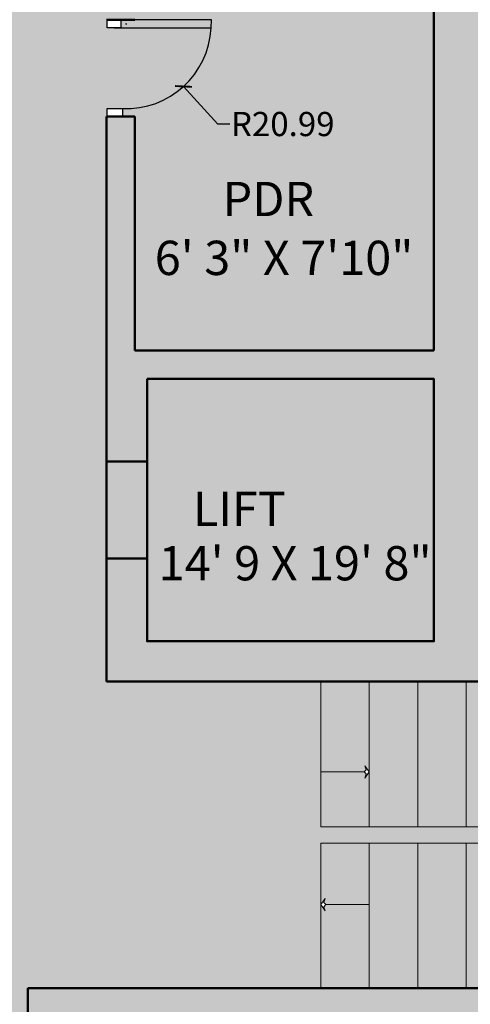
# Model space of a CAD drawing. Units: inches. Extents: x 925 to 2834, y 111 to 1355.
# Tile 7 of 25: x 1490 to 1602, y 638 to 882. Entities that reach past the tile are written whole.
import ezdxf

# ---------------------------------------------------------------- set-up
doc = ezdxf.new("R2010")
doc.units = ezdxf.units.IN
doc.header["$MEASUREMENT"] = 0
for name, color, linetype, lineweight in [('A-ANNO-DIMS', 2, 'Continuous', 18), ('A-AREA-IDEN', 7, 'Continuous', 18), ('A-DOOR', 2, 'Continuous', 25), ('A-FLOR-PATT', 252, 'Continuous', 13), ('A-FLOR-STRS', 4, 'Continuous', 18), ('A-WALL', 7, 'Continuous', 50), ('A-WALL-PATT', 8, 'Continuous', 13)]:
    doc.layers.add(name, color=color, linetype=linetype, lineweight=lineweight)
doc.styles.get("Standard").update_dxf_attribs({"font": 'arial.ttf'})
doc.dimstyles.get("Standard").update_dxf_attribs({"dimtxt": 6, "dimasz": 3, "dimexe": 0.18, "dimexo": 0.0625, "dimgap": 0.09, "dimtad": 0, "dimtih": 1, "dimtoh": 1, "dimdec": 1, "dimzin": 0, "dimdsep": 46, "dimlunit": 3, "dimtxsty": 'Standard', "dimblk": 'ARCHTICK', "dimcen": 0.09, "dimadec": 0, "dimazin": 0, "dimtfac": 1, "dimtdec": 1, "dimtofl": 0, "dimtmove": 0, "dimatfit": 3, "dimfxl": 1, "dimtolj": 1, "dimtzin": 0, "dimarcsym": 0})

# ---------------------------------------------------------------- blocks, each defined once
blk = doc.blocks.new('_ArchTick')
at = {"color": 0, "linetype": 'ByBlock', "const_width": 0.15}
blk.add_lwpolyline([(-0.5, -0.5), (0.5, 0.5)], dxfattribs=at)
blk = doc.blocks.new('*D83')
at = {"layer": 'A-ANNO-DIMS', "color": 0, "lineweight": -2, "transparency": 16777216}
for p, q in [((1516.5, 880.55), (1516.68, 880.55)), ((1516.59, 880.46), (1516.59, 880.64)), ((1539.21, 855.74), (1530.73, 865.05)), ((1542.21, 855.74), (1539.21, 855.74))]:
    blk.add_line(p, q, dxfattribs=at)
at = {"layer": 'Defpoints', "color": 0, "transparency": 16777216}
for p in [(1516.59, 880.55), (1530.73, 865.05)]:
    blk.add_point(p, dxfattribs=at)
at = {"layer": 'A-ANNO-DIMS', "color": 0, "lineweight": -2, "transparency": 16777216, "xscale": 3, "yscale": 3, "zscale": 3, "rotation": 132.3610318704431}
blk.add_blockref('_ArchTick', (1530.73, 865.05), dxfattribs=at)
at = {"layer": 'A-ANNO-DIMS', "color": 0, "transparency": 16777216, "insert": (1555.3, 855.74), "char_height": 6, "attachment_point": 5}
blk.add_mtext('\\A1;R20.99', dxfattribs=at)

msp = doc.modelspace()

# ---------------------------------------------------------------- hatches: boundary and pattern name
at = {"layer": 'A-FLOR-PATT', "transparency": 33554605}
h = msp.add_hatch(color=256, dxfattribs=at)
h.dxf.hatch_style = 1
h.paths.add_polyline_path([(1931.688, 1294.5638), (991.7375, 1294.5638), (991.7375, 172.1134), (1931.688, 172.1134)])
h.paths.add_polyline_path([(1910.7128, 1273.5886), (1910.7128, 193.0886), (1012.7128, 193.0886), (1012.7128, 1273.5886)], flags=16)
h.paths.add_polyline_path([(1850.7128, 1213.5886), (1850.7128, 253.0886), (1072.7128, 253.0886), (1072.7128, 1213.5886)], flags=0)
h.paths.add_polyline_path([(1838.7128, 1201.5886), (1838.7128, 265.0886), (1084.7128, 265.0886), (1084.7128, 530.5886), (1084.7128, 1201.5886)], flags=0)
h.paths.add_polyline_path([(1547.6758, 1155.7396), (1547.6758, 1119.115), (1513.0687, 1119.115), (1513.0687, 1155.7396)], flags=0)
h.paths.add_polyline_path([(1600.1067, 1154.9439), (1634.7139, 1154.9439), (1634.7139, 1119.115), (1600.1067, 1119.115)], flags=0)
h.paths.add_polyline_path([(1505.2502, 1144.5358), (1505.2502, 1119.115), (1470.643, 1119.115), (1470.643, 1144.5358)], flags=0)
h.paths.add_polyline_path([(1559.1357, 1141.0962), (1593.7428, 1141.0962), (1593.7428, 1119.115), (1559.1357, 1119.115)], flags=0)
h.paths.add_polyline_path([(1462.8966, 1154.9439), (1462.8966, 1119.115), (1428.2895, 1119.115), (1428.2895, 1154.9439)], flags=0)
h.paths.add_polyline_path([(1642.4603, 1144.5358), (1677.0675, 1144.5358), (1677.0675, 1119.115), (1642.4603, 1119.115)], flags=0)
h.paths.add_polyline_path([(1422.3508, 1141.0962), (1422.3508, 1119.115), (1387.7436, 1119.115), (1387.7436, 1141.0962)], flags=0)
h.paths.add_polyline_path([(1684.8859, 1155.7396), (1719.4931, 1155.7396), (1719.4931, 1119.115), (1684.8859, 1119.115)], flags=0)
h.paths.add_polyline_path([(1718.7128, 1081.5886), (1718.7128, 1050.1249), (1715.7128, 1050.1249), (1715.7128, 1026.1249), (1715.7128, 1002.1249), (1718.7128, 1002.1249), (1730.7128, 1002.1249), (1730.7128, 998.1249), (1730.7128, 990.1249), (1730.7128, 986.1249), (1718.7128, 986.1249), (1718.7128, 893.5886), (1715.3735, 893.5886), (1715.3735, 891.5886), (1713.3735, 891.5886, 0.41421356), (1677.3735, 855.5886), (1713.3735, 855.5886), (1713.3735, 853.5886), (1715.3735, 853.5886), (1715.3735, 851.5886), (1718.7128, 851.5886), (1718.7128, 821.5865), (1734.4655, 821.5865), (1734.3735, 819.5886, -0.41421356), (1712.4415, 793.5886), (1712.4415, 791.5886), (1718.7128, 791.5886), (1718.7128, 717.5886), (1718.7128, 669.5886), (1732.7128, 669.5886), (1732.7128, 665.5886), (1732.7128, 641.5886), (1732.7128, 634.5886), (1732.7128, 610.5886), (1732.7128, 603.5886), (1718.7128, 603.5886), (1718.7128, 385.0886), (1434.2128, 385.0886), (1434.2128, 530.5886), (1410.2128, 530.5886), (1408.2128, 530.5886), (1408.2128, 532.5886, 0.41421356), (1372.2128, 568.5886), (1372.2128, 532.5886), (1370.2128, 532.5886), (1370.2128, 530.5886), (1368.2128, 530.5886), (1282.2128, 530.5886), (1210.2128, 530.5886), (1200.2128, 530.5886), (1200.2128, 542.1915), (1183.2307, 542.1915), (1183.2307, 546.1915), (1200.2128, 546.1915), (1200.2128, 572.1915), (1183.2307, 572.1915), (1183.2307, 576.1915), (1200.2128, 576.1915), (1200.2128, 727.5886), (1210.2128, 727.5886), (1234.2128, 727.5886), (1259.7128, 727.5886), (1259.7128, 775.5886), (1259.7128, 799.5886), (1259.7128, 847.5886), (1259.7128, 993.5872), (1259.7128, 1065.5872), (1259.7128, 1071.5886), (1219.6318, 1071.5886), (1219.6318, 1081.5886), (1084.7128, 1081.5886), (1084.7128, 1119.115), (1256.8974, 1119.115), (1256.8974, 1154.9439), (1291.5046, 1154.9439), (1291.5046, 1119.115), (1256.8974, 1119.115), (1256.6723, 1081.5886), (1293.7128, 1081.5886), (1341.7128, 1081.5886), (1341.7128, 1093.5886), (1347.7128, 1093.5886), (1371.7128, 1093.5886), (1377.7128, 1093.5886), (1377.7128, 1081.5886), (1668.7128, 1081.5886), (1668.7128, 1117.5886), (1675.7128, 1117.5886), (1711.7128, 1117.5886), (1718.7128, 1117.5886)], flags=0)
h.paths.add_polyline_path([(1376.2838, 1155.7396), (1376.2838, 1119.115), (1341.6766, 1119.115), (1341.6766, 1155.7396)], flags=0)
h.paths.add_polyline_path([(1341.7128, 1076.0886), (1293.7128, 1076.0886), (1293.7128, 1071.5886), (1269.7128, 1071.5886), (1269.7128, 1065.5872), (1266.7128, 1065.5872), (1266.7128, 1029.5872), (1265.7128, 1029.5872), (1265.7128, 993.5872), (1269.7128, 993.5872), (1269.7128, 903.5886), (1269.7128, 893.5886), (1269.7128, 847.5886), (1265.2128, 847.5886), (1265.2128, 799.5886), (1269.7128, 799.5886), (1269.7128, 775.5886), (1265.2128, 775.5886), (1265.2128, 727.5886), (1269.7128, 727.5886), (1444.2128, 727.5886), (1444.2128, 717.5886), (1234.2128, 717.5886), (1234.2128, 722.0886), (1210.2128, 722.0886), (1210.2128, 717.5886), (1210.2128, 540.5886), (1210.2128, 536.0886), (1282.2128, 536.0886), (1282.2128, 535.0886), (1210.2128, 535.0886), (1210.2128, 540.5886), (1210.2128, 717.5886), (1210.2128, 723.0886), (1234.2128, 723.0886), (1234.2128, 717.5886), (1444.2128, 717.5886), (1444.2128, 727.5886), (1269.7128, 727.5886), (1264.2128, 727.5886), (1264.2128, 775.5886), (1269.7128, 775.5886), (1269.7128, 799.5886), (1264.2128, 799.5886), (1264.2128, 847.5886), (1269.7128, 847.5886), (1269.7128, 893.5886), (1269.7128, 903.5886), (1269.7128, 993.5872), (1264.7128, 993.5872), (1264.7128, 1029.5872), (1265.7128, 1029.5872), (1265.7128, 1065.5872), (1269.7128, 1065.5872), (1269.7128, 1071.5886), (1293.7128, 1071.5886), (1293.7128, 1077.0886), (1341.7128, 1077.0886)], flags=0)
h.paths.add_polyline_path([(1730.9529, 1141.0962), (1765.5601, 1141.0962), (1765.5601, 1119.115), (1730.9529, 1119.115)], flags=0)
h.paths.add_polyline_path([(1333.8582, 1144.5358), (1333.8582, 1119.115), (1299.251, 1119.115), (1299.251, 1144.5358)], flags=0)
h.paths.add_polyline_path([(1592.7128, 968.5886), (1596.0342, 968.5886), (1602.7128, 968.5886), (1708.7128, 968.5886), (1708.7128, 903.5886), (1602.7128, 903.5886), (1602.7128, 938.5886), (1592.7128, 938.5886), (1592.7128, 903.5886), (1451.7128, 903.5886), (1451.7128, 893.5886), (1511.7128, 893.5886), (1511.7128, 881.5886), (1515.2128, 881.5886), (1518.7128, 881.5886), (1518.7128, 893.5886), (1592.7128, 893.5886), (1592.7128, 799.5886), (1518.7128, 799.5886), (1518.7128, 857.5886), (1511.7128, 857.5886), (1511.7128, 799.5886), (1511.7128, 772.0886), (1521.7128, 772.0886), (1521.7128, 792.5886), (1592.7128, 792.5886), (1592.7128, 727.5886), (1521.7128, 727.5886), (1521.7128, 748.0886), (1511.7128, 748.0886), (1511.7128, 717.5886), (1708.7128, 717.5886), (1714.2128, 717.5886), (1714.2128, 669.5886), (1708.7128, 669.5886), (1708.7128, 641.5886), (1492.2128, 641.5886), (1492.2128, 631.5886), (1621.2128, 631.5886), (1621.2128, 443.0886), (1625.7128, 443.0886), (1625.7128, 503.0886), (1625.7128, 507.5886), (1625.7128, 631.5886), (1708.7128, 631.5886), (1708.7128, 507.5886), (1655.7128, 507.5886), (1655.7128, 503.0886), (1708.7128, 503.0886), (1708.7128, 395.0886), (1625.7128, 395.0886), (1625.7128, 419.0886), (1621.2128, 419.0886), (1621.2128, 395.0886), (1482.2128, 395.0886), (1482.2128, 385.0886), (1434.2128, 385.0886), (1434.2128, 433.0886), (1444.2128, 433.0886), (1444.2128, 631.5886), (1450.2128, 631.5886), (1450.2128, 634.91), (1452.2128, 634.91), (1452.2128, 669.5886), (1454.2128, 669.5886, -0.40021217), (1490.1712, 635.3173), (1492.2128, 635.3173), (1492.2128, 641.5886), (1564.7128, 641.5886), (1564.7128, 677.5886), (1672.7128, 677.5886), (1672.7128, 681.5886), (1564.7128, 681.5886), (1564.7128, 717.5886), (1511.7128, 717.5886), (1511.7128, 748.0886), (1511.7128, 772.0886), (1511.7128, 799.5886), (1511.7128, 857.5886), (1511.8913, 857.5886), (1511.8913, 859.5886), (1515.6201, 859.5886, 0.41421356), (1537.552, 879.5886), (1513.552, 879.5886), (1511.8913, 879.5886), (1511.8913, 881.5886), (1511.7128, 881.5886), (1511.7128, 893.5886), (1451.7128, 893.5886), (1451.7128, 903.5886), (1592.7128, 903.5886), (1592.7128, 938.5886), (1592.7128, 940.5886), (1596.4415, 940.5886, 0.41421356), (1618.3735, 966.5886), (1594.3735, 966.5886), (1592.7128, 966.5886)], flags=0)
h.paths.add_polyline_path([(1377.7128, 903.5886), (1377.7128, 893.5886), (1305.7128, 893.5886), (1305.7128, 903.5886)], flags=0)
h.paths.add_polyline_path([(1708.7128, 821.5886), (1712.0342, 821.5886), (1712.0342, 819.5886), (1710.3735, 819.5886), (1708.7128, 819.5886)], flags=0)
h.paths.add_polyline_path([(1576.7128, 695.1992), (1575.5896, 693.6649), (1575.9687, 694.6994), (1575.4438, 695.1992), (1575.9687, 695.699), (1575.5896, 696.7335)], flags=0)
h.paths.add_polyline_path([(1565.9817, 662.3134), (1565.4568, 661.8136), (1565.8359, 660.7791), (1564.7128, 662.3134), (1565.8359, 663.8477), (1565.4568, 662.8132)], flags=0)
h.paths.add_polyline_path([(1444.2128, 433.0886), (1444.2128, 395.0886), (1482.2128, 395.0886), (1482.2128, 389.0886), (1438.2128, 389.0886), (1438.2128, 391.8608), (1438.2128, 433.0886)], flags=0)
h.paths.add_polyline_path([(1410.2128, 506.5886), (1410.2128, 289.0886), (1108.7128, 289.0886), (1108.7128, 506.5886)], flags=0)
h.paths.add_polyline_path([(1612.3153, 838.3016), (1680.4151, 838.3016), (1680.4151, 851.3131), (1612.3153, 851.3131)], flags=8)
h.paths.add_polyline_path([(1208.3174, 395.0436), (1282.1017, 395.0436), (1282.1017, 408.0552), (1208.3174, 408.0552)], flags=8)
h.paths.add_polyline_path([(1291.8049, 598.7427), (1369.8017, 598.7427), (1369.8017, 611.7542), (1291.8049, 611.7542)], flags=8)
h.paths.add_polyline_path([(1119.679, 917.3022), (1191.0817, 917.3022), (1191.0817, 930.3137), (1119.679, 930.3137)], flags=8)
h.paths.add_polyline_path([(1332.2261, 815.9808), (1410.2258, 815.9808), (1410.2258, 829.001), (1332.2261, 829.001)], flags=8)
h.paths.add_polyline_path([(1390.9013, 955.8158), (1475.4981, 955.8158), (1475.4981, 968.8273), (1390.9013, 968.8273)], flags=8)
h.paths.add_polyline_path([(1620.3436, 998.9325), (1688.4434, 998.9325), (1688.4434, 1011.944), (1620.3436, 1011.944)], flags=8)
h.paths.add_polyline_path([(1620.3436, 914.1039), (1691.7405, 914.1039), (1691.7405, 927.1155), (1620.3436, 927.1155)], flags=8)
h.paths.add_polyline_path([(1521.4542, 816.005), (1589.5569, 816.005), (1589.5569, 829.0253), (1521.4542, 829.0253)], flags=8)
h.paths.add_polyline_path([(1528.524, 740.3497), (1602.3082, 740.3497), (1602.3082, 753.3613), (1528.524, 753.3613)], flags=8)
h.paths.add_polyline_path([(1627.6094, 762.6128), (1702.3091, 762.6128), (1702.3091, 775.6244), (1627.6094, 775.6244)], flags=8)
h.paths.add_polyline_path([(1610.5442, 657.2751), (1684.3284, 657.2751), (1684.3284, 670.2867), (1610.5442, 670.2867)], flags=8)
h.paths.add_polyline_path([(1636.6983, 519.472), (1711.3981, 519.472), (1711.3981, 532.4835), (1636.6983, 532.4835)], flags=8)
h.paths.add_polyline_path([(1616.8577, 424.8539), (1694.8545, 424.8539), (1694.8545, 437.8654), (1616.8577, 437.8654)], flags=8)
h.paths.add_polyline_path([(1506.1456, 460.8838), (1579.9299, 460.8838), (1579.9299, 473.8953), (1506.1456, 473.8953)], flags=8)
h.paths.add_polyline_path([(1624.6119, 784.6011), (1696.9185, 784.6011), (1696.9185, 797.7864), (1624.6119, 797.7864)], flags=8)
h.paths.add_polyline_path([(1606.3732, 854.2194), (1683.3039, 854.2194), (1683.3039, 867.4048), (1606.3732, 867.4048)], flags=8)
h.paths.add_polyline_path([(1127.8008, 940.3581), (1165.1637, 940.3581), (1165.1637, 953.5348), (1127.8008, 953.5348)], flags=8)
h.paths.add_polyline_path([(1620.8657, 1019.4968), (1677.3447, 1019.4968), (1677.3447, 1032.6735), (1620.8657, 1032.6735)], flags=8)
h.paths.add_polyline_path([(1620.8643, 930.1821), (1703.0564, 930.1821), (1703.0564, 943.3675), (1620.8643, 943.3675)], flags=8)
h.paths.add_polyline_path([(1324.5702, 836.8338), (1408.0892, 836.8338), (1408.0892, 850.0191), (1324.5702, 850.0191)], flags=8)
h.paths.add_polyline_path([(1281.6584, 622.8885), (1383.6213, 622.8885), (1383.6213, 636.0739), (1281.6584, 636.0739)], flags=8)
h.paths.add_polyline_path([(1210.6721, 416.7893), (1269.1299, 416.7893), (1269.1299, 429.9747), (1210.6721, 429.9747)], flags=8)
h.paths.add_polyline_path([(1507.8264, 477.4836), (1586.7329, 477.4836), (1586.7329, 490.669), (1507.8264, 490.669)], flags=8)
h.paths.add_polyline_path([(1643.6238, 443.8135), (1696.6696, 443.8135), (1696.6696, 456.5643), (1643.6238, 456.5643)], flags=8)
h.paths.add_polyline_path([(1647.2466, 540.5638), (1693.1825, 540.5638), (1693.1825, 553.7491), (1647.2466, 553.7491)], flags=8)
h.paths.add_polyline_path([(1626.0633, 668.5064), (1673.3174, 668.5064), (1673.3174, 681.6831), (1626.0633, 681.6831)], flags=8)
h.paths.add_polyline_path([(1538.2915, 830.7872), (1567.5942, 830.7872), (1567.5942, 843.5293), (1538.2915, 843.5293)], flags=8)
h.paths.add_polyline_path([(1530.9338, 754.0477), (1559.576, 754.0477), (1559.576, 766.7898), (1530.9338, 766.7898)], flags=8)
h.paths.add_polyline_path([(1351.2461, 979.2309), (1513.8919, 979.2309), (1513.8919, 992.4076), (1351.2461, 992.4076)], flags=8)
at = {"layer": 'A-FLOR-PATT'}
h = msp.add_hatch(color=256, dxfattribs=at)
h.dxf.hatch_style = 1
h.paths.add_polyline_path([(1850.7128, 1213.5886), (1072.7128, 1213.5886), (1072.7128, 253.0886), (1850.7128, 253.0886)])
h.paths.add_polyline_path([(1084.7128, 1201.5886), (1838.7128, 1201.5886), (1838.7128, 265.0886), (1084.7128, 265.0886)], flags=16)
h.paths.add_polyline_path([(1183.2307, 576.1915), (1200.2128, 576.1915), (1200.2128, 727.5886), (1210.2128, 727.5886), (1234.2128, 727.5886), (1259.7128, 727.5886), (1259.7128, 775.5886), (1259.7128, 799.5886), (1259.7128, 847.5886), (1259.7128, 993.5872), (1259.7128, 1065.5872), (1259.7128, 1071.5886), (1219.6318, 1071.5886), (1219.6318, 1081.5886), (1293.7128, 1081.5886), (1341.7128, 1081.5886), (1341.7128, 1093.5886), (1347.7128, 1093.5886), (1347.7128, 1081.5886), (1371.7128, 1081.5886), (1371.7128, 1093.5886), (1377.7128, 1093.5886), (1377.7128, 1081.5886), (1668.7128, 1081.5886), (1668.7128, 1117.5886), (1675.7128, 1117.5886), (1675.7128, 1081.5886), (1711.7128, 1081.5886), (1711.7128, 1117.5886), (1718.7128, 1117.5886), (1718.7128, 1081.5886), (1718.7128, 1050.1249), (1715.7128, 1050.1249), (1715.7128, 1026.1249), (1715.7128, 1002.1249), (1718.7128, 1002.1249), (1730.7128, 1002.1249), (1730.7128, 998.1249), (1730.7128, 990.1249), (1730.7128, 986.1249), (1718.7128, 986.1249), (1718.7128, 893.5886), (1715.3735, 893.5886), (1715.3735, 891.5886), (1713.3735, 891.5886, 0.41421356), (1677.3735, 855.5886), (1713.3735, 855.5886), (1713.3735, 853.5886), (1715.3735, 853.5886), (1715.3735, 851.5886), (1718.7128, 851.5886), (1718.7128, 821.5865), (1734.4655, 821.5865), (1734.3735, 819.5886, -0.41421356), (1712.4415, 793.5886), (1712.4415, 791.5886), (1718.7128, 791.5886), (1718.7128, 717.5886), (1718.7128, 669.5886), (1732.7128, 669.5886), (1732.7128, 665.5886), (1732.7128, 641.5886), (1732.7128, 634.5886), (1732.7128, 610.5886), (1732.7128, 603.5886), (1718.7128, 603.5886), (1718.7128, 385.0886), (1434.2128, 385.0886), (1434.2128, 433.0886), (1434.2128, 530.5886), (1410.2128, 530.5886), (1408.2128, 530.5886), (1408.2128, 532.5886, 0.41421356), (1372.2128, 568.5886), (1372.2128, 532.5886), (1370.2128, 532.5886), (1370.2128, 530.5886), (1368.2128, 530.5886), (1282.2128, 530.5886), (1210.2128, 530.5886), (1200.2128, 530.5886), (1200.2128, 542.1915), (1183.2307, 542.1915), (1183.2307, 546.1915), (1200.2128, 546.1915), (1200.2128, 572.1915), (1183.2307, 572.1915)], flags=0)
h.paths.add_polyline_path([(1210.2128, 717.5886), (1210.2128, 723.0886), (1234.2128, 723.0886), (1234.2128, 717.5886), (1444.2128, 717.5886), (1444.2128, 727.5886), (1269.7128, 727.5886), (1264.2128, 727.5886), (1264.2128, 775.5886), (1269.7128, 775.5886), (1269.7128, 799.5886), (1264.2128, 799.5886), (1264.2128, 847.5886), (1269.7128, 847.5886), (1269.7128, 893.5886), (1269.7128, 903.5886), (1269.7128, 993.5872), (1264.7128, 993.5872), (1264.7128, 1029.5872), (1265.7128, 1029.5872), (1265.7128, 1065.5872), (1269.7128, 1065.5872), (1269.7128, 1071.5886), (1293.7128, 1071.5886), (1293.7128, 1077.0886), (1341.7128, 1077.0886), (1341.7128, 1076.0886), (1293.7128, 1076.0886), (1293.7128, 1071.5886), (1269.7128, 1071.5886), (1269.7128, 1065.5872), (1266.7128, 1065.5872), (1266.7128, 1029.5872), (1265.7128, 1029.5872), (1265.7128, 993.5872), (1269.7128, 993.5872), (1269.7128, 903.5886), (1269.7128, 893.5886), (1269.7128, 847.5886), (1265.2128, 847.5886), (1265.2128, 799.5886), (1269.7128, 799.5886), (1269.7128, 775.5886), (1265.2128, 775.5886), (1265.2128, 727.5886), (1269.7128, 727.5886), (1444.2128, 727.5886), (1444.2128, 717.5886), (1234.2128, 717.5886), (1234.2128, 722.0886), (1210.2128, 722.0886), (1210.2128, 717.5886), (1210.2128, 540.5886), (1210.2128, 536.0886), (1282.2128, 536.0886), (1282.2128, 535.0886), (1210.2128, 535.0886), (1210.2128, 540.5886)], flags=0)
h.paths.add_polyline_path([(1450.2128, 634.91), (1452.2128, 634.91), (1452.2128, 669.5886), (1454.2128, 669.5886, -0.40021217), (1490.1712, 635.3173), (1492.2128, 635.3173), (1492.2128, 641.5886), (1564.7128, 641.5886), (1564.7128, 677.5886), (1672.7128, 677.5886), (1672.7128, 681.5886), (1564.7128, 681.5886), (1564.7128, 717.5886), (1511.7128, 717.5886), (1511.7128, 748.0886), (1511.7128, 772.0886), (1511.7128, 799.5886), (1511.7128, 857.5886), (1511.8913, 857.5886), (1511.8913, 859.5886), (1515.6201, 859.5886, 0.41421356), (1537.552, 879.5886), (1513.552, 879.5886), (1511.8913, 879.5886), (1511.8913, 881.5886), (1511.7128, 881.5886), (1511.7128, 893.5886), (1451.7128, 893.5886), (1451.7128, 903.5886), (1592.7128, 903.5886), (1592.7128, 938.5886), (1592.7128, 940.5886), (1596.4415, 940.5886, 0.41421356), (1618.3735, 966.5886), (1594.3735, 966.5886), (1592.7128, 966.5886), (1592.7128, 968.5886), (1596.0342, 968.5886), (1602.7128, 968.5886), (1708.7128, 968.5886), (1708.7128, 903.5886), (1602.7128, 903.5886), (1602.7128, 938.5886), (1592.7128, 938.5886), (1592.7128, 903.5886), (1451.7128, 903.5886), (1451.7128, 893.5886), (1511.7128, 893.5886), (1511.7128, 881.5886), (1518.7128, 881.5886), (1518.7128, 893.5886), (1592.7128, 893.5886), (1592.7128, 799.5886), (1518.7128, 799.5886), (1518.7128, 857.5886), (1511.7128, 857.5886), (1511.7128, 799.5886), (1511.7128, 772.0886), (1521.7128, 772.0886), (1521.7128, 792.5886), (1592.7128, 792.5886), (1592.7128, 727.5886), (1521.7128, 727.5886), (1521.7128, 748.0886), (1511.7128, 748.0886), (1511.7128, 717.5886), (1708.7128, 717.5886), (1714.2128, 717.5886), (1714.2128, 669.5886), (1708.7128, 669.5886), (1708.7128, 641.5886), (1492.2128, 641.5886), (1492.2128, 631.5886), (1621.2128, 631.5886), (1621.2128, 443.0886), (1625.7128, 443.0886), (1625.7128, 503.0886), (1625.7128, 507.5886), (1625.7128, 631.5886), (1708.7128, 631.5886), (1708.7128, 507.5886), (1655.7128, 507.5886), (1655.7128, 503.0886), (1708.7128, 503.0886), (1708.7128, 395.0886), (1625.7128, 395.0886), (1625.7128, 419.0886), (1621.2128, 419.0886), (1621.2128, 395.0886), (1482.2128, 395.0886), (1482.2128, 389.0886), (1438.2128, 389.0886), (1438.2128, 391.8608), (1438.2128, 433.0886), (1444.2128, 433.0886), (1444.2128, 631.5886), (1450.2128, 631.5886)], flags=0)
h.paths.add_polyline_path([(1444.2128, 433.0886), (1444.2128, 395.0886), (1482.2128, 395.0886), (1482.2128, 391.0886), (1440.2128, 391.0886), (1440.2128, 391.8608), (1440.2128, 433.0886)], flags=0)
h.paths.add_polyline_path([(1305.7128, 893.5886), (1305.7128, 903.5886), (1377.7128, 903.5886), (1377.7128, 893.5886)], flags=0)
h.paths.add_polyline_path([(1564.7128, 662.3134), (1565.8359, 663.8477), (1565.4568, 662.8132), (1565.9817, 662.3134), (1565.4568, 661.8136), (1565.8359, 660.7791)], flags=0)
h.paths.add_polyline_path([(1575.4438, 695.1992), (1575.9687, 695.699), (1575.5896, 696.7335), (1576.7128, 695.1992), (1575.5896, 693.6649), (1575.9687, 694.6994)], flags=0)
h.paths.add_polyline_path([(1708.7128, 821.5886), (1712.0342, 821.5886), (1712.0342, 819.5886), (1710.3735, 819.5886), (1708.7128, 819.5886)], flags=0)
h = msp.add_hatch(color=256, dxfattribs=at)
h.dxf.hatch_style = 1
h.paths.add_polyline_path([(1718.7128, 603.5886), (1708.7128, 603.5886), (1708.7128, 507.5886), (1655.7128, 507.5886), (1655.7128, 503.0886), (1708.7128, 503.0886), (1708.7128, 395.0886), (1625.7128, 395.0886), (1625.7128, 419.0886), (1621.2128, 419.0886), (1621.2128, 395.0886), (1482.2128, 395.0886), (1482.2128, 385.0886), (1718.7128, 385.0886)])
h.paths.add_polyline_path([(1625.7128, 631.5886), (1708.7128, 631.5886), (1708.7128, 603.5886), (1718.7128, 603.5886), (1732.7128, 603.5886), (1732.7128, 610.5886), (1715.7128, 610.5886), (1715.7128, 634.5886), (1732.7128, 634.5886), (1732.7128, 641.5886), (1715.7128, 641.5886), (1715.7128, 665.5886), (1732.7128, 665.5886), (1732.7128, 669.5886), (1708.7128, 669.5886), (1708.7128, 641.5886), (1492.2128, 641.5886), (1492.2128, 631.5886), (1621.2128, 631.5886), (1621.2128, 443.0886), (1625.7128, 443.0886), (1625.7128, 503.0886), (1625.7128, 507.5886)])
h.paths.add_polyline_path([(1718.7128, 851.5886), (1708.7128, 851.5886), (1708.7128, 828.5886), (1602.7128, 828.5886), (1602.7128, 893.5886), (1708.7128, 893.5886), (1718.7128, 893.5886), (1718.7128, 986.1249), (1730.7128, 986.1249), (1730.7128, 990.1249), (1718.7128, 990.1249), (1718.7128, 998.1249), (1730.7128, 998.1249), (1730.7128, 1002.1249), (1718.7128, 1002.1249), (1708.7128, 1002.1249), (1708.7128, 975.5886), (1602.7128, 975.5886), (1602.7128, 1011.5886), (1592.7128, 1011.5886), (1592.7128, 968.5886), (1596.0342, 968.5886), (1602.7128, 968.5886), (1708.7128, 968.5886), (1708.7128, 903.5886), (1602.7128, 903.5886), (1602.7128, 938.5886), (1592.7128, 938.5886), (1592.7128, 903.5886), (1451.7128, 903.5886), (1451.7128, 893.5886), (1511.7128, 893.5886), (1511.7128, 881.5886), (1515.2128, 881.5886), (1518.7128, 881.5886), (1518.7128, 893.5886), (1592.7128, 893.5886), (1592.7128, 799.5886), (1518.7128, 799.5886), (1518.7128, 857.5886), (1511.7128, 857.5886), (1511.7128, 799.5886), (1511.7128, 772.0886), (1521.7128, 772.0886), (1521.7128, 792.5886), (1592.7128, 792.5886), (1592.7128, 727.5886), (1521.7128, 727.5886), (1521.7128, 748.0886), (1511.7128, 748.0886), (1511.7128, 717.5886), (1708.7128, 717.5886), (1718.7128, 717.5886), (1718.7128, 727.5886), (1718.7128, 791.5886), (1708.7128, 791.5886), (1708.7128, 727.5886), (1602.7128, 727.5886), (1602.7128, 821.5886), (1708.7128, 821.5886), (1712.0342, 821.5886), (1718.7128, 821.5886)])
h.paths.add_polyline_path([(1718.7128, 1081.5886), (1718.7128, 1117.5886), (1711.7128, 1117.5886), (1711.7128, 1081.5886), (1675.7128, 1081.5886), (1675.7128, 1117.5886), (1668.7128, 1117.5886), (1668.7128, 1081.5886), (1377.7128, 1081.5886), (1377.7128, 1093.5886), (1371.7128, 1093.5886), (1371.7128, 1081.5886), (1347.7128, 1081.5886), (1347.7128, 1093.5886), (1341.7128, 1093.5886), (1341.7128, 1081.5886), (1341.7128, 1071.5886), (1592.7128, 1071.5886), (1592.7128, 1035.5886), (1602.7128, 1035.5886), (1602.7128, 1071.5886), (1708.7128, 1071.5886), (1708.7128, 1050.1249), (1718.7128, 1050.1249)])
h.paths.add_polyline_path([(1293.7128, 1081.5886), (1219.6318, 1081.5886), (1219.6318, 1071.5886), (1259.7128, 1071.5886), (1259.7128, 1065.5872), (1269.7128, 1065.5872), (1269.7128, 1071.5886), (1293.7128, 1071.5886)])
h.paths.add_polyline_path([(1269.7128, 903.5886), (1269.7128, 993.5872), (1259.7128, 993.5872), (1259.7128, 847.5886), (1269.7128, 847.5886), (1269.7128, 893.5886)])
h.paths.add_polyline_path([(1377.7128, 903.5886), (1305.7128, 903.5886), (1305.7128, 893.5886), (1377.7128, 893.5886)])
h.paths.add_polyline_path([(1444.2128, 727.5886), (1269.7128, 727.5886), (1259.7128, 727.5886), (1234.2128, 727.5886), (1234.2128, 717.5886), (1444.2128, 717.5886)])
h.paths.add_polyline_path([(1269.7128, 799.5886), (1259.7128, 799.5886), (1259.7128, 775.5886), (1269.7128, 775.5886)])
h.paths.add_polyline_path([(1444.2128, 631.5886), (1450.2128, 631.5886), (1450.2128, 634.91), (1450.2128, 641.5886), (1434.2128, 641.5886), (1434.2128, 540.5886), (1410.2128, 540.5886), (1410.2128, 530.5886), (1434.2128, 530.5886), (1434.2128, 433.0886), (1444.2128, 433.0886)])
h.paths.add_polyline_path([(1368.2128, 533.91), (1368.2128, 540.5886), (1282.2128, 540.5886), (1282.2128, 530.5886), (1368.2128, 530.5886)])
h.paths.add_polyline_path([(1210.2128, 717.5886), (1210.2128, 727.5886), (1200.2128, 727.5886), (1200.2128, 576.1915), (1183.2307, 576.1915), (1183.2307, 572.1915), (1200.2128, 572.1915), (1200.2128, 546.1915), (1183.2307, 546.1915), (1183.2307, 542.1915), (1200.2128, 542.1915), (1200.2128, 530.5886), (1210.2128, 530.5886), (1210.2128, 540.5886)])
at = {"layer": 'A-FLOR-PATT', "transparency": 33554605}
h = msp.add_hatch(color=256, dxfattribs=at)
h.dxf.hatch_style = 1
h.paths.add_polyline_path([(1592.7128, 938.5886), (1592.7128, 940.5886), (1596.4415, 940.5886, 0.41421356), (1618.3735, 966.5886), (1594.3735, 966.5886), (1592.7128, 966.5886), (1592.7128, 968.5886), (1592.7128, 1011.5886), (1602.7128, 1011.5886), (1602.7128, 975.5886), (1708.7128, 975.5886), (1708.7128, 1002.1249), (1711.7128, 1002.1249), (1711.7128, 1026.1249), (1711.7128, 1050.1249), (1708.7128, 1050.1249), (1708.7128, 1071.5886), (1602.7128, 1071.5886), (1602.7128, 1035.5886), (1592.7128, 1035.5886), (1592.7128, 1071.5886), (1341.7128, 1071.5886), (1293.7128, 1071.5886), (1269.7128, 1071.5886), (1269.7128, 1065.5872), (1269.7128, 993.5872), (1269.7128, 903.5886), (1269.7128, 893.5886), (1269.7128, 847.5886), (1269.7128, 799.5886), (1269.7128, 775.5886), (1269.7128, 727.5886), (1444.2128, 727.5886), (1444.2128, 717.5886), (1234.2128, 717.5886), (1210.2128, 717.5886), (1210.2128, 540.5886), (1282.2128, 540.5886), (1368.2128, 540.5886), (1368.2128, 533.91), (1370.2128, 533.91), (1370.2128, 568.5886), (1372.2128, 568.5886, -0.40021217), (1408.1712, 534.3173), (1410.2128, 534.3173), (1410.2128, 540.5886), (1434.2128, 540.5886), (1434.2128, 641.5886), (1450.2128, 641.5886), (1450.2128, 634.91), (1452.2128, 634.91), (1452.2128, 669.5886), (1454.2128, 669.5886, -0.40021217), (1490.1712, 635.3173), (1492.2128, 635.3173), (1492.2128, 641.5886), (1564.7128, 641.5886), (1564.7128, 677.5886), (1672.7128, 677.5886), (1672.7128, 681.5886), (1564.7128, 681.5886), (1564.7128, 717.5886), (1511.7128, 717.5886), (1511.7128, 748.0886), (1511.7128, 772.0886), (1511.7128, 799.5886), (1511.7128, 857.5886), (1511.8913, 857.5886), (1511.8913, 859.5886), (1515.6201, 859.5886, 0.41421356), (1537.552, 879.5886), (1513.552, 879.5886), (1511.8913, 879.5886), (1511.8913, 881.5886), (1511.7128, 881.5886), (1511.7128, 893.5886), (1451.7128, 893.5886), (1451.7128, 903.5886), (1592.7128, 903.5886)])
h.paths.add_polyline_path([(1377.7128, 903.5886), (1377.7128, 893.5886), (1305.7128, 893.5886), (1305.7128, 903.5886)], flags=16)
h.paths.add_polyline_path([(1592.7128, 893.5886), (1518.7128, 893.5886), (1518.7128, 881.5865), (1537.6441, 881.5865), (1537.552, 879.5886, -0.41421356), (1515.6201, 859.5886), (1515.6201, 857.5886), (1518.7128, 857.5886), (1518.7128, 799.5886), (1592.7128, 799.5886)], flags=17)
h.paths.add_polyline_path([(1291.8049, 598.7427), (1369.8017, 598.7427), (1369.8017, 611.7542), (1291.8049, 611.7542)], flags=24)
h.paths.add_polyline_path([(1332.2261, 815.9808), (1410.2258, 815.9808), (1410.2258, 829.001), (1332.2261, 829.001)], flags=24)
h.paths.add_polyline_path([(1390.9013, 955.8158), (1475.4981, 955.8158), (1475.4981, 968.8273), (1390.9013, 968.8273)], flags=24)
h.paths.add_polyline_path([(1620.3436, 998.9325), (1688.4434, 998.9325), (1688.4434, 1011.944), (1620.3436, 1011.944)], flags=24)
h.paths.add_polyline_path([(1620.8657, 1019.4968), (1677.3447, 1019.4968), (1677.3447, 1032.6735), (1620.8657, 1032.6735)], flags=24)
h.paths.add_polyline_path([(1324.5702, 836.8338), (1408.0892, 836.8338), (1408.0892, 850.0191), (1324.5702, 850.0191)], flags=24)
h.paths.add_polyline_path([(1281.6584, 622.8885), (1383.6213, 622.8885), (1383.6213, 636.0739), (1281.6584, 636.0739)], flags=24)
h.paths.add_polyline_path([(1626.0633, 668.5064), (1673.3174, 668.5064), (1673.3174, 681.6831), (1626.0633, 681.6831)], flags=25)
h.paths.add_polyline_path([(1351.2461, 979.2309), (1513.8919, 979.2309), (1513.8919, 992.4076), (1351.2461, 992.4076)], flags=24)
h.paths.add_polyline_path([(1521.4542, 816.005), (1589.5569, 816.005), (1589.5569, 829.0253), (1521.4542, 829.0253)], flags=24)
h.paths.add_polyline_path([(1538.2915, 830.7872), (1567.5942, 830.7872), (1567.5942, 843.5293), (1538.2915, 843.5293)], flags=24)
h.paths.add_polyline_path([(1636.6983, 519.472), (1711.3981, 519.472), (1711.3981, 532.4835), (1636.6983, 532.4835)], flags=9)
h.paths.add_polyline_path([(1616.8577, 424.8539), (1694.8545, 424.8539), (1694.8545, 437.8654), (1616.8577, 437.8654)], flags=9)
h.paths.add_polyline_path([(1506.1456, 460.8838), (1579.9299, 460.8838), (1579.9299, 473.8953), (1506.1456, 473.8953)], flags=9)
h.paths.add_polyline_path([(1606.3732, 854.2194), (1683.3039, 854.2194), (1683.3039, 867.4048), (1606.3732, 867.4048)], flags=25)
h.paths.add_polyline_path([(1507.8264, 477.4836), (1586.7329, 477.4836), (1586.7329, 490.669), (1507.8264, 490.669)], flags=9)
h.paths.add_polyline_path([(1643.6238, 443.8135), (1696.6696, 443.8135), (1696.6696, 456.5643), (1643.6238, 456.5643)], flags=9)
h.paths.add_polyline_path([(1647.2466, 540.5638), (1693.1825, 540.5638), (1693.1825, 553.7491), (1647.2466, 553.7491)], flags=25)
h = msp.add_hatch(color=256, dxfattribs=at)
h.dxf.hatch_style = 1
h.paths.add_polyline_path([(1200.2128, 727.5886), (1084.7128, 727.5886), (1084.7128, 530.5886), (1200.2128, 530.5886), (1200.2128, 542.1915), (1183.2307, 542.1915), (1183.2307, 546.1915), (1200.2128, 546.1915), (1200.2128, 572.1915), (1183.2307, 572.1915), (1183.2307, 576.1915), (1200.2128, 576.1915)])
h.paths.add_polyline_path([(1612.3153, 838.3016), (1680.4151, 838.3016), (1680.4151, 851.3131), (1612.3153, 851.3131)], flags=9)
h.paths.add_polyline_path([(1291.8049, 598.7427), (1369.8017, 598.7427), (1369.8017, 611.7542), (1291.8049, 611.7542)], flags=9)
h.paths.add_polyline_path([(1119.679, 917.3022), (1191.0817, 917.3022), (1191.0817, 930.3137), (1119.679, 930.3137)], flags=9)
h.paths.add_polyline_path([(1332.2261, 815.9808), (1410.2258, 815.9808), (1410.2258, 829.001), (1332.2261, 829.001)], flags=9)
h.paths.add_polyline_path([(1390.9013, 955.8158), (1475.4981, 955.8158), (1475.4981, 968.8273), (1390.9013, 968.8273)], flags=9)
h.paths.add_polyline_path([(1620.3436, 998.9325), (1688.4434, 998.9325), (1688.4434, 1011.944), (1620.3436, 1011.944)], flags=9)
h.paths.add_polyline_path([(1620.3436, 914.1039), (1691.7405, 914.1039), (1691.7405, 927.1155), (1620.3436, 927.1155)], flags=9)
h.paths.add_polyline_path([(1521.4542, 816.005), (1589.5569, 816.005), (1589.5569, 829.0253), (1521.4542, 829.0253)], flags=9)
h.paths.add_polyline_path([(1522.4337, 740.3497), (1596.218, 740.3497), (1596.218, 753.3613), (1522.4337, 753.3613)], flags=9)
h.paths.add_polyline_path([(1606.3732, 854.2194), (1683.3039, 854.2194), (1683.3039, 867.4048), (1606.3732, 867.4048)], flags=9)
h.paths.add_polyline_path([(1127.8008, 940.3581), (1165.1637, 940.3581), (1165.1637, 953.5348), (1127.8008, 953.5348)], flags=9)
h.paths.add_polyline_path([(1620.8657, 1019.4968), (1677.3447, 1019.4968), (1677.3447, 1032.6735), (1620.8657, 1032.6735)], flags=9)
h.paths.add_polyline_path([(1620.8643, 930.1821), (1703.0564, 930.1821), (1703.0564, 943.3675), (1620.8643, 943.3675)], flags=9)
h.paths.add_polyline_path([(1324.5702, 836.8338), (1408.0892, 836.8338), (1408.0892, 850.0191), (1324.5702, 850.0191)], flags=9)
h.paths.add_polyline_path([(1281.6584, 622.8885), (1383.6213, 622.8885), (1383.6213, 636.0739), (1281.6584, 636.0739)], flags=9)
h.paths.add_polyline_path([(1626.0633, 668.5064), (1673.3174, 668.5064), (1673.3174, 681.6831), (1626.0633, 681.6831)], flags=9)
h.paths.add_polyline_path([(1538.2915, 830.7872), (1567.5942, 830.7872), (1567.5942, 843.5293), (1538.2915, 843.5293)], flags=9)
h.paths.add_polyline_path([(1351.2461, 979.2309), (1513.8919, 979.2309), (1513.8919, 992.4076), (1351.2461, 992.4076)], flags=9)
h = msp.add_hatch(color=256, dxfattribs=at)
h.dxf.hatch_style = 1
h.paths.add_polyline_path([(1621.2128, 631.5886), (1492.2128, 631.5886), (1490.2128, 631.5886), (1490.2128, 633.5886, 0.41421356), (1454.2128, 669.5886), (1454.2128, 633.5886), (1452.2128, 633.5886), (1452.2128, 631.5886), (1450.2128, 631.5886), (1444.2128, 631.5886), (1444.2128, 395.0886), (1482.2128, 395.0886), (1621.2128, 395.0886), (1621.2128, 419.0886), (1625.7128, 419.0886), (1625.7128, 395.0886), (1708.7128, 395.0886), (1708.7128, 503.0886), (1655.7128, 503.0886), (1655.7128, 507.5886), (1708.7128, 507.5886), (1708.7128, 631.5886), (1625.7128, 631.5886), (1625.7128, 507.5886), (1625.7128, 503.0886), (1625.7128, 443.0886), (1621.2128, 443.0886)])
h.paths.add_polyline_path([(1636.6983, 519.472), (1711.3981, 519.472), (1711.3981, 532.4835), (1636.6983, 532.4835)], flags=9)
h.paths.add_polyline_path([(1616.8577, 424.8539), (1694.8545, 424.8539), (1694.8545, 437.8654), (1616.8577, 437.8654)], flags=24)
h.paths.add_polyline_path([(1506.1456, 460.8838), (1579.9299, 460.8838), (1579.9299, 473.8953), (1506.1456, 473.8953)], flags=24)
h.paths.add_polyline_path([(1507.8264, 477.4836), (1586.7329, 477.4836), (1586.7329, 490.669), (1507.8264, 490.669)], flags=24)
h.paths.add_polyline_path([(1643.6238, 443.8135), (1696.6696, 443.8135), (1696.6696, 456.5643), (1643.6238, 456.5643)], flags=24)
h.paths.add_polyline_path([(1647.2466, 540.5638), (1693.1825, 540.5638), (1693.1825, 553.7491), (1647.2466, 553.7491)], flags=24)
h.paths.add_polyline_path([(1612.3153, 838.3016), (1680.4151, 838.3016), (1680.4151, 851.3131), (1612.3153, 851.3131)], flags=9)
h.paths.add_polyline_path([(1291.8049, 598.7427), (1369.8017, 598.7427), (1369.8017, 611.7542), (1291.8049, 611.7542)], flags=9)
h.paths.add_polyline_path([(1119.679, 917.3022), (1191.0817, 917.3022), (1191.0817, 930.3137), (1119.679, 930.3137)], flags=9)
h.paths.add_polyline_path([(1332.2261, 815.9808), (1410.2258, 815.9808), (1410.2258, 829.001), (1332.2261, 829.001)], flags=9)
h.paths.add_polyline_path([(1390.9013, 955.8158), (1475.4981, 955.8158), (1475.4981, 968.8273), (1390.9013, 968.8273)], flags=9)
h.paths.add_polyline_path([(1620.3436, 998.9325), (1688.4434, 998.9325), (1688.4434, 1011.944), (1620.3436, 1011.944)], flags=9)
h.paths.add_polyline_path([(1620.3436, 914.1039), (1691.7405, 914.1039), (1691.7405, 927.1155), (1620.3436, 927.1155)], flags=9)
h.paths.add_polyline_path([(1521.4542, 816.005), (1589.5569, 816.005), (1589.5569, 829.0253), (1521.4542, 829.0253)], flags=9)
h.paths.add_polyline_path([(1528.524, 740.3497), (1602.3082, 740.3497), (1602.3082, 753.3613), (1528.524, 753.3613)], flags=9)
h.paths.add_polyline_path([(1627.6094, 762.6128), (1702.3091, 762.6128), (1702.3091, 775.6244), (1627.6094, 775.6244)], flags=9)
h.paths.add_polyline_path([(1624.6119, 784.6011), (1696.9185, 784.6011), (1696.9185, 797.7864), (1624.6119, 797.7864)], flags=9)
h.paths.add_polyline_path([(1606.3732, 854.2194), (1683.3039, 854.2194), (1683.3039, 867.4048), (1606.3732, 867.4048)], flags=9)
h.paths.add_polyline_path([(1127.8008, 940.3581), (1165.1637, 940.3581), (1165.1637, 953.5348), (1127.8008, 953.5348)], flags=9)
h.paths.add_polyline_path([(1620.8657, 1019.4968), (1677.3447, 1019.4968), (1677.3447, 1032.6735), (1620.8657, 1032.6735)], flags=9)
h.paths.add_polyline_path([(1620.8643, 930.1821), (1703.0564, 930.1821), (1703.0564, 943.3675), (1620.8643, 943.3675)], flags=9)
h.paths.add_polyline_path([(1324.5702, 836.8338), (1408.0892, 836.8338), (1408.0892, 850.0191), (1324.5702, 850.0191)], flags=9)
h.paths.add_polyline_path([(1281.6584, 622.8885), (1383.6213, 622.8885), (1383.6213, 636.0739), (1281.6584, 636.0739)], flags=9)
h.paths.add_polyline_path([(1626.0633, 668.5064), (1673.3174, 668.5064), (1673.3174, 681.6831), (1626.0633, 681.6831)], flags=9)
h.paths.add_polyline_path([(1538.2915, 830.7872), (1567.5942, 830.7872), (1567.5942, 843.5293), (1538.2915, 843.5293)], flags=9)
h.paths.add_polyline_path([(1530.9338, 754.0477), (1559.576, 754.0477), (1559.576, 766.7898), (1530.9338, 766.7898)], flags=9)
h.paths.add_polyline_path([(1351.2461, 979.2309), (1513.8919, 979.2309), (1513.8919, 992.4076), (1351.2461, 992.4076)], flags=9)
h = msp.add_hatch(color=256, dxfattribs=at)
h.dxf.hatch_style = 1
h.paths.add_polyline_path([(1708.7128, 791.5886), (1708.7128, 793.5886), (1712.4415, 793.5886, 0.41421356), (1734.3735, 819.5886), (1710.3735, 819.5886), (1708.7128, 819.5886), (1708.7128, 821.5886), (1602.7128, 821.5886), (1602.7128, 727.5886), (1708.7128, 727.5886)])
h.paths.add_polyline_path([(1708.7128, 851.5886), (1712.052, 851.5886), (1712.052, 853.5886), (1677.3735, 853.5886), (1677.3735, 855.5886, -0.40021217), (1711.6447, 891.5471), (1711.6447, 893.5886), (1708.7128, 893.5886), (1602.7128, 893.5886), (1602.7128, 828.5886), (1708.7128, 828.5886)])
h.paths.add_polyline_path([(1708.7128, 968.5886), (1618.4656, 968.5886), (1618.3735, 966.5886, -0.41421356), (1596.4415, 940.5886), (1596.4415, 938.5886), (1602.7128, 938.5886), (1602.7128, 903.5886), (1708.7128, 903.5886)])
h.paths.add_polyline_path([(1708.7128, 717.5886), (1672.7128, 717.5886), (1672.7128, 641.5886), (1708.7128, 641.5886)])
h.paths.add_polyline_path([(1588.7128, 717.5886), (1576.7128, 717.5886), (1576.7128, 681.5886), (1588.7128, 681.5886)])
h.paths.add_polyline_path([(1576.7128, 717.5886), (1564.7128, 717.5886), (1564.7128, 695.1992), (1575.4438, 695.1992), (1575.9687, 695.699), (1575.5896, 696.7335), (1576.7128, 695.1992)])
h.paths.add_polyline_path([(1576.7128, 695.1992), (1575.5896, 693.6649), (1575.9687, 694.6994), (1575.4438, 695.1992), (1564.7128, 695.1992), (1564.7128, 681.5886), (1576.7128, 681.5886)])
h.paths.add_polyline_path([(1600.7128, 717.5886), (1588.7128, 717.5886), (1588.7128, 681.5886), (1600.7128, 681.5886)])
h.paths.add_polyline_path([(1612.7128, 717.5886), (1600.7128, 717.5886), (1600.7128, 681.5886), (1612.7128, 681.5886)])
h.paths.add_polyline_path([(1624.7128, 717.5886), (1612.7128, 717.5886), (1612.7128, 681.5886), (1624.7128, 681.5886)])
h.paths.add_polyline_path([(1636.7128, 717.5886), (1624.7128, 717.5886), (1624.7128, 681.5886), (1636.7128, 681.5886)])
h.paths.add_polyline_path([(1648.7128, 717.5886), (1636.7128, 717.5886), (1636.7128, 681.5886), (1648.7128, 681.5886)])
h.paths.add_polyline_path([(1660.7128, 717.5886), (1648.7128, 717.5886), (1648.7128, 681.5886), (1660.7128, 681.5886)])
h.paths.add_polyline_path([(1672.7128, 717.5886), (1660.7128, 717.5886), (1660.7128, 681.5886), (1672.7128, 681.5886)])
h.paths.add_polyline_path([(1576.7128, 662.3134), (1565.9817, 662.3134), (1565.4568, 661.8136), (1565.8359, 660.7791), (1564.7128, 662.3134), (1564.7128, 641.5886), (1576.7128, 641.5886)])
h.paths.add_polyline_path([(1576.7128, 677.5886), (1564.7128, 677.5886), (1564.7128, 662.3134), (1565.8359, 663.8477), (1565.4568, 662.8132), (1565.9817, 662.3134), (1576.7128, 662.3134)])
h.paths.add_polyline_path([(1588.7128, 677.5886), (1576.7128, 677.5886), (1576.7128, 641.5886), (1588.7128, 641.5886)])
h.paths.add_polyline_path([(1600.7128, 677.5886), (1588.7128, 677.5886), (1588.7128, 641.5886), (1600.7128, 641.5886)])
h.paths.add_polyline_path([(1612.7128, 677.5886), (1600.7128, 677.5886), (1600.7128, 641.5886), (1612.7128, 641.5886)])
h.paths.add_polyline_path([(1624.7128, 677.5886), (1612.7128, 677.5886), (1612.7128, 641.5886), (1624.7128, 641.5886)])
h.paths.add_polyline_path([(1636.7128, 677.5886), (1624.7128, 677.5886), (1624.7128, 641.5886), (1636.7128, 641.5886)])
h.paths.add_polyline_path([(1648.7128, 677.5886), (1636.7128, 677.5886), (1636.7128, 641.5886), (1648.7128, 641.5886)])
h.paths.add_polyline_path([(1660.7128, 677.5886), (1648.7128, 677.5886), (1648.7128, 641.5886), (1660.7128, 641.5886)])
h.paths.add_polyline_path([(1672.7128, 677.5886), (1660.7128, 677.5886), (1660.7128, 641.5886), (1672.7128, 641.5886)])
h.paths.add_polyline_path([(1627.6094, 762.6128), (1702.3091, 762.6128), (1702.3091, 775.6244), (1627.6094, 775.6244)], flags=24)
h.paths.add_polyline_path([(1624.6119, 784.6011), (1696.9185, 784.6011), (1696.9185, 797.7864), (1624.6119, 797.7864)], flags=24)
h.paths.add_polyline_path([(1612.3153, 838.3016), (1680.4151, 838.3016), (1680.4151, 851.3131), (1612.3153, 851.3131)], flags=24)
h.paths.add_polyline_path([(1606.3732, 854.2194), (1683.3039, 854.2194), (1683.3039, 867.4048), (1606.3732, 867.4048)], flags=24)
h.paths.add_polyline_path([(1620.3436, 914.1039), (1691.7405, 914.1039), (1691.7405, 927.1155), (1620.3436, 927.1155)], flags=24)
h.paths.add_polyline_path([(1620.8643, 930.1821), (1703.0564, 930.1821), (1703.0564, 943.3675), (1620.8643, 943.3675)], flags=24)
h.paths.add_polyline_path([(1610.5442, 657.2751), (1684.3284, 657.2751), (1684.3284, 670.2867), (1610.5442, 670.2867)], flags=9)
h.paths.add_polyline_path([(1626.0633, 668.5064), (1673.3174, 668.5064), (1673.3174, 681.6831), (1626.0633, 681.6831)], flags=9)
at = {"layer": 'A-FLOR-PATT'}
h = msp.add_hatch(color=256, dxfattribs=at)
h.dxf.hatch_style = 1
h.paths.add_polyline_path([(1713.3735, 855.5886), (1677.3735, 855.5886), (1677.3735, 853.5886), (1713.3735, 853.5886)])
h.paths.add_polyline_path([(1372.2128, 568.5886), (1370.2128, 568.5886), (1370.2128, 532.5886), (1372.2128, 532.5886)])
h.paths.add_polyline_path([(1734.4655, 821.5865), (1712.0342, 821.5865), (1712.0342, 819.5886), (1734.3735, 819.5886)])
h.paths.add_polyline_path([(1454.2128, 669.5886), (1452.2128, 669.5886), (1452.2128, 633.5886), (1454.2128, 633.5886)])
h.paths.add_polyline_path([(1537.6441, 881.5865), (1515.2128, 881.5865), (1515.2128, 879.5886), (1537.552, 879.5886)])
at = {"layer": 'A-FLOR-PATT', "transparency": 33554605}
h = msp.add_hatch(color=256, dxfattribs=at)
h.dxf.hatch_style = 1
h.paths.add_polyline_path([(1592.7128, 792.5886), (1521.7128, 792.5886), (1521.7128, 727.5886), (1592.7128, 727.5886)])
h.paths.add_polyline_path([(1522.4337, 740.3497), (1596.218, 740.3497), (1596.218, 753.3613), (1522.4337, 753.3613)], flags=9)
h.paths.add_polyline_path([(1530.9338, 754.0477), (1559.576, 754.0477), (1559.576, 766.7898), (1530.9338, 766.7898)], flags=24)
at = {"layer": 'A-WALL-PATT'}
h = msp.add_hatch(color=256, dxfattribs=at)
h.dxf.hatch_style = 1
h.set_gradient(color1=(255, 255, 255), tint=1)
h.paths.add_polyline_path([(1521.7128, 748.0886), (1521.7128, 772.0886), (1511.7128, 772.0886), (1511.7128, 748.0886)])

# ---------------------------------------------------------------- linework, layer by layer
at = {"layer": 'A-DOOR'}
for p, q in [((1537.6441, 881.5865), (1515.2128, 881.5865)), ((1537.552, 879.5886), (1537.6441, 881.5865)), ((1513.552, 879.5886), (1537.552, 879.5886))]:
    msp.add_line(p, q, dxfattribs=at)
for points in [[(1515.2128, 881.5886), (1515.2128, 879.5886), (1511.8913, 879.5886), (1511.8913, 881.5886)], [(1515.6201, 859.5886), (1515.6201, 857.5886), (1511.8913, 857.5886), (1511.8913, 859.5886)]]:
    msp.add_lwpolyline(points, close=True, dxfattribs=at)
msp.add_arc((1516.586, 880.5546), 20.9882, 267.36202, 357.36202, dxfattribs=at)
at = {"layer": 'A-FLOR-STRS'}
for p, q in [((1564.7128, 681.5886), (1564.7128, 717.5886)), ((1576.7128, 681.5886), (1576.7128, 717.5886)), ((1588.7128, 681.5886), (1588.7128, 717.5886)), ((1600.7128, 681.5886), (1600.7128, 717.5886)), ((1575.9687, 695.699), (1575.4438, 695.1992)), ((1576.7128, 695.1992), (1575.5896, 696.7335)), ((1575.5896, 696.7335), (1575.9687, 695.699)), ((1564.7128, 695.1992), (1575.4438, 695.1992)), ((1575.9687, 694.6994), (1575.4438, 695.1992)), ((1576.7128, 695.1992), (1575.5896, 693.6649)), ((1575.5896, 693.6649), (1575.9687, 694.6994)), ((1672.7128, 681.5886), (1564.7128, 681.5886)), ((1564.7128, 641.5886), (1564.7128, 677.5886)), ((1672.7128, 677.5886), (1564.7128, 677.5886)), ((1576.7128, 641.5886), (1576.7128, 677.5886)), ((1588.7128, 641.5886), (1588.7128, 677.5886)), ((1600.7128, 641.5886), (1600.7128, 677.5886)), ((1564.7128, 662.3134), (1565.8359, 663.8477)), ((1565.8359, 663.8477), (1565.4568, 662.8132)), ((1564.7128, 662.3134), (1565.8359, 660.7791)), ((1565.4568, 662.8132), (1565.9817, 662.3134)), ((1565.4568, 661.8136), (1565.9817, 662.3134)), ((1565.8359, 660.7791), (1565.4568, 661.8136)), ((1576.7128, 662.3134), (1565.9817, 662.3134))]:
    msp.add_line(p, q, dxfattribs=at)
at = {"layer": 'A-WALL'}
for p, q in [((1592.7128, 893.5886), (1592.7128, 799.5886)), ((1518.7128, 881.5886), (1511.7128, 881.5886)), ((1518.7128, 857.5886), (1511.7128, 857.5886)), ((1511.7128, 857.5886), (1511.7128, 799.5886)), ((1518.7128, 857.5886), (1518.7128, 799.5886)), ((1511.7128, 799.5886), (1511.7128, 772.0886)), ((1518.7128, 799.5886), (1592.7128, 799.5886)), ((1521.7128, 792.5886), (1521.7128, 772.0886)), ((1521.7128, 792.5886), (1592.7128, 792.5886)), ((1592.7128, 792.5886), (1592.7128, 727.5886)), ((1521.7128, 772.0886), (1511.7128, 772.0886)), ((1521.7128, 748.0886), (1511.7128, 748.0886)), ((1511.7128, 748.0886), (1511.7128, 717.5886)), ((1521.7128, 748.0886), (1521.7128, 727.5886)), ((1592.7128, 727.5886), (1521.7128, 727.5886)), ((1708.7128, 717.5886), (1511.7128, 717.5886)), ((1708.7128, 641.5886), (1492.2128, 641.5886)), ((1492.2128, 631.5886), (1492.2128, 641.5886))]:
    msp.add_line(p, q, dxfattribs=at)
for points in [[(1521.7128, 792.5886), (1592.7128, 792.5886), (1592.7128, 727.5886), (1521.7128, 727.5886)], [(1521.7128, 772.0886), (1521.7128, 748.0886), (1511.7128, 748.0886), (1511.7128, 772.0886)]]:
    msp.add_lwpolyline(points, close=True, dxfattribs=at)

# ---------------------------------------------------------------- texts
at = {"layer": 'A-AREA-IDEN'}
for s, height, p in [('PDR', 8.49473, (1540.4151, 832.9108)), ('6\' 3" X 7\'10"', 8.494735, (1523.6242, 818.3257)), ('LIFT', 8.49473, (1533.0575, 756.1713)), ('14\' 9 X 19\' 8"', 8.494735, (1524.6023, 742.6632))]:
    msp.add_text(s, height=height, dxfattribs=at).set_placement(p)

# ---------------------------------------------------------------- dimensions: what is measured, and where the dimension line sits
at = {"layer": 'A-ANNO-DIMS'}
dim = msp.add_radius_dim(center=(1516.586, 880.5546), mpoint=(1530.7279, 865.0461), dimstyle='Standard', override={"dimdec": 2, "dimlfac": 1, "dimrnd": 0, "dimzin": 0, "dimdsep": 46, "dimlunit": 2}, dxfattribs=at)
dim.commit()
dim.dimension.update_dxf_attribs({"geometry": '*D83', "text_midpoint": (1555.3037, 855.741), "dimtype": 164})

doc.saveas('drawing.dxf')
